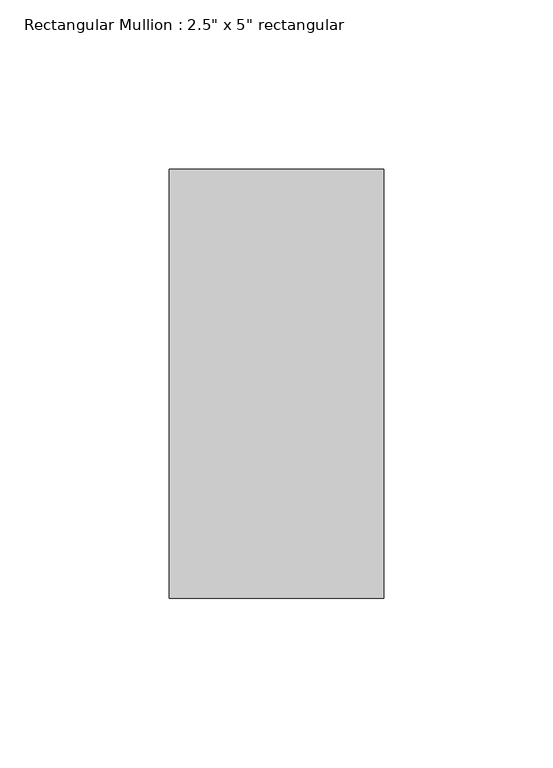
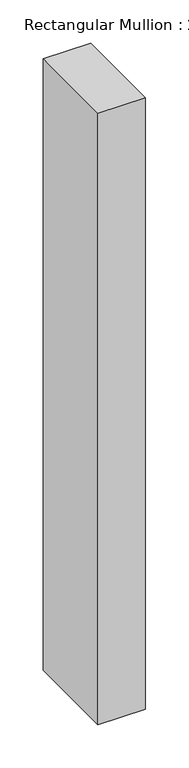
"""IFC4 building model written with IfcOpenShell, lengths in millimetres: member geometry."""

from ifc_helpers import new_model, si_unit, frame, origin, place, context, project, spatial, polyline, outline, extrude, source, transform, mapped, element, save


def member_b00ab025(model_context):
    return source(origin(), model_context, "Body", "SweptSolid", [
        extrude(outline(polyline([(31.75, 63.5), (31.75, -63.5), (-31.75, -63.5), (-31.75, 63.5), (31.75, 63.5)])), frame((0.0, 0.0, -864.6440196), z_axis=(0.0, 0.0, 1.0), x_axis=(1.0, 0.0, 0.0)), (0.0, 0.0, 1.0), 864.6440196),
    ])


if __name__ == "__main__":
    model = new_model("IFC4")
    model_context = context("Model", 3, world=origin())
    ifc_project = project(units=[si_unit("LENGTHUNIT", "METRE", prefix="MILLI")], contexts=[model_context])
    site = spatial("IfcSite", under=ifc_project)
    building = spatial("IfcBuilding", under=site)
    placement = place(None, origin())
    member_shape = member_b00ab025(model_context)
    element("IfcMember", 1, ObjectType="Rectangular Mullion : 2.5\" x 5\" rectangular", at=placement, inside=building, context=model_context, shape_type="MappedRepresentation", body=[
        mapped(member_shape, transform((0.0, 0.0, 0.0), x_axis=(1.0, 0.0, 0.0), y_axis=(0.0, 1.0, 0.0), z_axis=(0.0, 0.0, 1.0))),
    ])
    save(model, "model.ifc")

# Revit data of these elements
# Type "Rectangular Mullion : 2.5\" x 5\" rectangular"
#   built-in parameter 1007304 = 0.416667 (stored number, unit not read)
#   built-in parameter 1007301 = 0.104167 (stored number, unit not read)
#   built-in parameter 1007300 = 0.104167 (stored number, unit not read)
# Element 1 (IfcMember, "Rectangular Mullion : 2.5\" x 5\" rectangular")
#   Materials on its faces: "Aluminum"
# Materials
#   "Aluminum": class "Metal", colour RGB 247 247 247, transparency 0, Description = "Aluminum 6061", Cost = 0
